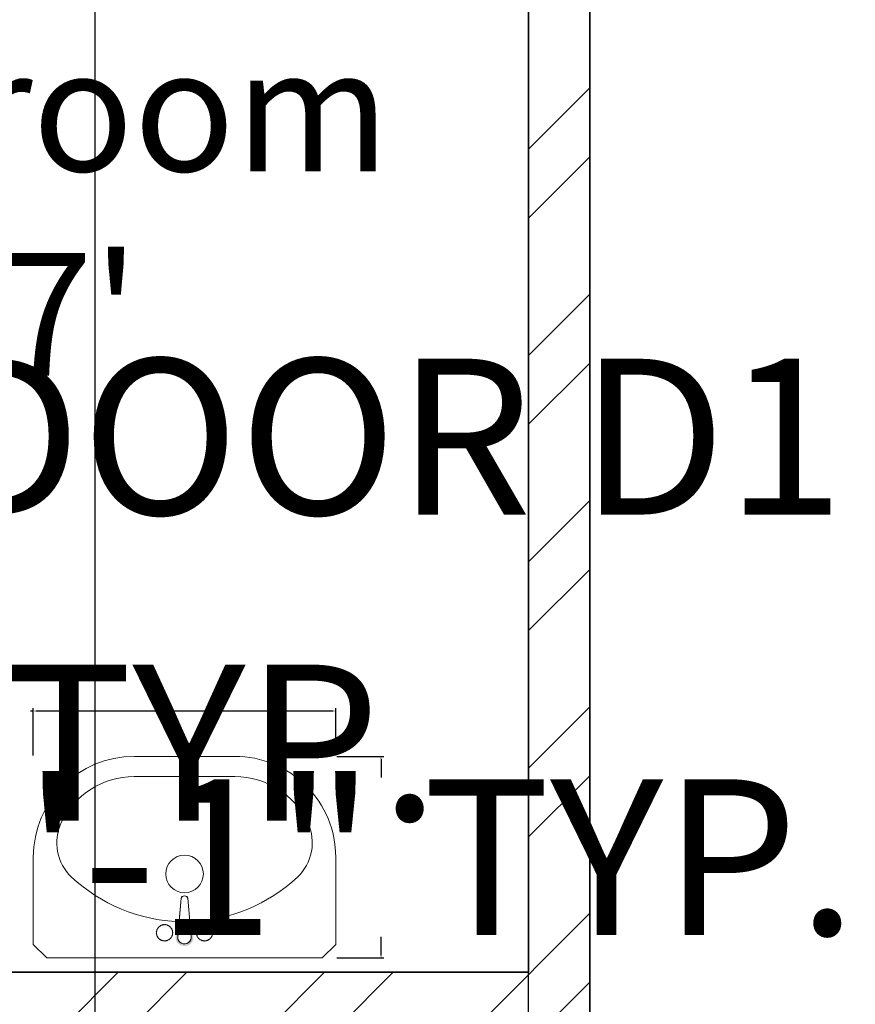
# Model space of a CAD drawing. Units: inches. Extents: x 2379 to 3013, y 1431 to 2110.
# Tile 7 of 10: x 2730 to 2785, y 1927 to 1991. Entities that reach past the tile are written whole.
import ezdxf

# ---------------------------------------------------------------- set-up
doc = ezdxf.new("R2010")
doc.units = ezdxf.units.IN
for name, color, linetype, lineweight in [('A-ANNO-DIMS', 2, 'Continuous', 18), ('A-AREA-IDEN', 7, 'Continuous', 18), ('A-FLOR-FIXT', 9, 'Continuous', 18), ('A-WALL-PATT', 8, 'Continuous', 13), ('WALL', 7, 'Continuous', 35)]:
    doc.layers.add(name, color=color, linetype=linetype, lineweight=lineweight)
doc.styles.get("Standard").update_dxf_attribs({"font": 'arial.ttf'})
doc.dimstyles.get("Standard").update_dxf_attribs({"dimtxt": 10.18, "dimasz": 0.18, "dimexe": 0.18, "dimexo": 0.0625, "dimgap": 0.09, "dimtad": 0, "dimtih": 1, "dimtoh": 1, "dimdec": 0, "dimzin": 0, "dimdsep": 46, "dimlunit": 3, "dimtxsty": 'Standard', "dimcen": 0.09, "dimadec": 0, "dimazin": 0, "dimtfac": 1, "dimtdec": 0, "dimtofl": 0, "dimtmove": 0, "dimatfit": 3, "dimfxl": 1, "dimtolj": 1, "dimtzin": 0, "dimarcsym": 0})

# ---------------------------------------------------------------- blocks, each defined once
blk = doc.blocks.new('s_46')
at = {"ltscale": 600}
h = blk.add_hatch(color=256, dxfattribs=at)
edge = h.paths.add_edge_path()
edge.add_line((13.45184378023259, 62.04360352296498), (14.15927104179718, 54.09782096462731))
edge.add_ellipse((4.212458010588306, 52.31250418393756), major_axis=(-10.10576298371302, 2.5e-15), ratio=1, start_angle=540, end_angle=550.1754626554052, ccw=False)
edge.add_arc((4.212458010588306, 52.31250418393756), 10.10576298371302, 270, 360, ccw=False)
edge.add_line((4.212458010588306, 42.20674120020703), (4.212458010588306, 41.28018079043977))
edge.add_line((4.212458010588306, 41.28018079040339), (11.85106942148559, 41.28018079040339))
edge.add_arc((4.212458010588306, 52.31250418393756), 13.41866400745597, 664.6981342835142, 766.4847699121552)
h.paths.add_polyline_path([(4.212458010588306, 41.28018079040339), (-3.426153400272596, 41.28018079040339, 0.152566653256377), (4.212458010588306, 38.8938401764608)])
h.paths.add_polyline_path([(11.85106942144921, 41.28018079040339), (4.212458010588306, 41.28018079040339), (4.212458010588306, 38.8938401764608, 0.1525666532563772)])
h.paths.add_polyline_path([(-5.734355020395014, 54.09782096461277), (-5.026927758881356, 62.04360352296498, 0.4758332592079194), (-3.426153400272596, 41.28018079040339), (4.212458010588306, 41.28018079040339), (4.212458010588306, 42.20674120020703, -0.4672400657637396)])
for p, q in [((-5.893304973142221, 52.31250418385025), (-0.714987907151226, 110.4750654234667)), ((-5.893304973142221, 52.31250418385025), (-0.714987907151226, 110.4750654234667)), ((9.139903928502463, 110.475065423554), (14.15927104174625, 54.09782096461277)), ((14.31822099431883, 52.31250418385025), (9.139903928502463, 110.475065423554)), ((14.15927104174625, 54.09782096461277), (14.31822099431883, 52.31250418385025))]:
    blk.add_line(p, q, dxfattribs=at)
blk.add_lwpolyline([(-220.7875419894117, 171.2801807903452, -0.4142135623730951), (-70.7875419894117, 321.2801807903452), (79.2124580105883, 321.2801807904325, -0.4142135623730951), (229.2124580105883, 171.2801807904325), (229.2124580105883, 41.28018079040339), (209.2124580107047, 21.2801807904325), (-200.7875419893535, 21.28018079034518), (-220.7875419894117, 41.28018079040339)], format="xyb", close=True, dxfattribs=at)
blk.add_lwpolyline([(12.26164246437838, 75.41187665969483, 0.1816379869150311), (172.1859176590806, 141.5383421540609, 0.3263505073803008), (187.6570333366981, 222.6589125997853, 0.2898144196813102), (79.21245801076293, 291.2801807904325), (-70.78754198923707, 291.2801807903452, 0.2898144196813102), (-179.2321173155214, 222.658912599698, 0.3263505073803008), (-163.7610016377293, 141.5383421540609, 0.1816379869150315), (-3.836726442852523, 75.41187665960751)], format="xyb", dxfattribs=at)
for points in [[(-16.83803374727722, 67.43055756771354), (-17.02338931558188, 67.50428807432763), (-17.22058725368697, 67.56961317334208), (-17.42189012444578, 67.6347039079701), (-17.61956049106084, 67.70773132116301), (-17.80586091603618, 67.79686645595939), (-17.97305396257434, 67.91028035557245), (-18.11578784312587, 68.05326030802098), (-18.23825336818117, 68.21955858168076), (-18.34702699835179, 68.40004368982045), (-18.44868519355077, 68.58558414605795), (-18.54980441438965, 68.76704846357461), (-18.65696112113073, 68.9353051558137), (-18.77673177386168, 69.08122273621848), (-18.91569283319404, 69.19566971814493), (-19.07841429975815, 69.27267628890695), (-19.26144033775199, 69.31891933156292), (-19.45930865121772, 69.34423740339116), (-19.66655694507062, 69.35846906132065), (-19.87772292352747, 69.37145286262967), (-20.08734429115429, 69.39302736415993), (-20.2899587523425, 69.43303112310241), (-20.48010401183274, 69.50130269664805), (-20.65391131333308, 69.60429419830325), (-20.81388605764368, 69.73491196823306), (-20.96412718523061, 69.8826759030926), (-21.10873363655992, 70.03710589953698), (-21.25180435174844, 70.18772185422131), (-21.39743827126222, 70.3240436638007), (-21.54973433539272, 70.43559122501756), (-21.71279148443137, 70.5118844343524), (-21.88955151231494, 70.54600451889564), (-22.07832762773614, 70.54527802669325), (-22.27627589285839, 70.52059283622657), (-22.4805523698451, 70.48283682571491), (-22.68831312085968, 70.44289787355228), (-22.89671420806553, 70.41166385821998), (-23.10291169380071, 70.40002265802468), (-23.30406164005399, 70.41886215136037), (-23.49802141042892, 70.4753938675276), (-23.68545357254334, 70.56212393892929), (-23.86772199510597, 70.66788214896224), (-24.04619054717477, 70.78149828102323), (-24.22222309763311, 70.89180211850908), (-24.39718351518968, 70.98762344472925), (-24.57243566872785, 71.05779204316786), (-24.74934342730558, 71.09113769704709), (-24.92903553397628, 71.08022740500746), (-25.11170022917213, 71.03257702605333), (-25.2972906283685, 70.95943963443278), (-25.48575984616764, 70.8720683044812), (-25.67706099752104, 70.7817161102721), (-25.87114719772944, 70.69963612605352), (-26.0679715613951, 70.63708142607356), (-26.26748720381875, 70.60530508466763), (-26.46941223740578, 70.61182491958607), (-26.67252476507565, 70.64921772302478), (-26.87536788737634, 70.70632503094384), (-27.07648470485583, 70.77198837930337), (-27.27441831788747, 70.8350493038015), (-27.46771182701923, 70.88434934031102), (-27.6549083327991, 70.90873002487933), (-27.83455093560042, 70.8970328932919), (-28.00620139669627, 70.84190539614065), (-28.17349611973623, 70.75121864315588), (-28.34109016874572, 70.63664965887438), (-28.51363860827405, 70.50987546765828), (-28.69579650234664, 70.38257309404435), (-28.89221891516354, 70.26641956248204), (-29.10756091127405, 70.17309189750813), (-29.3464775547036, 70.11426712348475), (-29.61160253512208, 70.0940409177856), (-29.89748404390411, 70.0861835690448), (-30.19664889771957, 70.05688401864609), (-30.50162391323829, 69.9723312081478), (-30.80493590747938, 69.79871407902101), (-31.09911169676343, 69.50222157256212), (-31.37667809793493, 69.0490426304168), (-31.63016192783834, 68.40536619405611), (-32.32050594605971, 68.4500712644367), (-32.84873653826071, 68.3918758847285), (-33.24226493795868, 68.25193804170704), (-33.52850237919483, 68.0514157223224), (-33.73486009566113, 67.8114669136994), (-33.88874932087492, 67.5532496026135), (-34.01758128887741, 67.29792177610216), (-34.14876723336056, 67.06664142102818), (-34.30371923936764, 66.87550954936887), (-34.47985279804561, 66.72039927294827), (-34.66858425136889, 66.59212672835565), (-34.86132994201034, 66.48150805244222), (-35.04950621211901, 66.37935938188457), (-35.22452940384392, 66.27649685335928), (-35.37781585985795, 66.16373660371755), (-35.50078192248475, 66.03189476963598), (-35.58785390376579, 65.87432967920904), (-35.64549799636007, 65.69456842611542), (-35.68319036299363, 65.49868029527715), (-35.7104071660433, 65.2927345718781), (-35.73662456823513, 65.08280054092756), (-35.77131873212056, 64.87494748734753), (-35.82396582007641, 64.67524469623459), (-35.90404199482873, 64.48976145259803), (-36.01774371694773, 64.3227640100813), (-36.15814863995183, 64.17130649695173), (-36.31505471485434, 64.0306400101108), (-36.47825989319244, 63.89601564637269), (-36.63756212632871, 63.76268450255157), (-36.78275936545106, 63.62589767554891), (-36.90364956192207, 63.48090626226621), (-36.99003066710429, 63.32296135951764), (-37.03518227743916, 63.14869254492805), (-37.04631056915969, 62.96024331927765), (-37.03410336375237, 62.7611356638954), (-37.00924848217983, 62.55489156045951), (-36.98243374592858, 62.34503299021162), (-36.96434697631048, 62.13508193491725), (-36.96567599463743, 61.92856037581805), (-36.99710862222128, 61.72899029450491), (-37.06570762058254, 61.53896291530691), (-37.16403551277472, 61.35734643402975), (-37.28102976223454, 61.18207828939194), (-37.40562783187488, 61.0110959201993), (-37.52676718513249, 60.84233676508302), (-37.63338528544409, 60.67373826284892), (-37.7144195958972, 60.50323785204091), (-37.75880757992855, 60.32877297155209), (-37.75920177751686, 60.14875038337777), (-37.72311503690435, 59.96345414296957), (-37.66177528270055, 59.77363762940512), (-37.58641044021351, 59.58005422132555), (-37.5082484340528, 59.38345729780849), (-37.43851718935184, 59.18460023758234), (-37.38844463089481, 58.98423641963745), (-37.36925868364051, 58.78311922278953), (-37.38844463089481, 58.58200202594161), (-37.43851718935184, 58.38163820799673), (-37.5082484340528, 58.18278114777058), (-37.58641044021351, 57.98618422425352), (-37.66177528287517, 57.79260081626126), (-37.72311503690435, 57.6027843026095), (-37.75920177751686, 57.4174880622013), (-37.75880757992855, 57.23746547402697), (-37.7144195958972, 57.06300059353816), (-37.63338528544409, 56.89250018273014), (-37.52676718530711, 56.72390168049606), (-37.40562783187488, 56.55514252537978), (-37.28102976223454, 56.38416015618713), (-37.16403551277472, 56.20889201154932), (-37.06570762058254, 56.02727553035947), (-36.99710862222128, 55.83724815107416), (-36.96567599463743, 55.63767806976102), (-36.96434697631048, 55.43115651066182), (-36.98243374592858, 55.22120545536745), (-37.00924848217983, 55.01134688520687), (-37.03410336375237, 54.80510278168367), (-37.04631056933431, 54.60599512638873), (-37.03518227743916, 54.41754590065102), (-36.99003066710429, 54.24327708606142), (-36.90364956192207, 54.08533218331285), (-36.78275936545106, 53.94034077003016), (-36.63756212632871, 53.80355394302751), (-36.47825989319244, 53.67022279920639), (-36.31505471502896, 53.53559843546827), (-36.15814863995183, 53.39493194862734), (-36.01774371712236, 53.24347443549777), (-35.90404199482873, 53.07647699298104), (-35.82396582007641, 52.89099374934449), (-35.77131873212056, 52.69129095823155), (-35.73662456823513, 52.48343790465151), (-35.71040716621792, 52.27350387370098), (-35.68319036299363, 52.06755815021461), (-35.64549799653469, 51.87167001946363), (-35.58785390376579, 51.69190876637003), (-35.50078192248475, 51.53434367594309), (-35.3778353385278, 51.40284301002975), (-35.22468523163116, 51.29247093791491), (-35.05003213009331, 51.19609060572111), (-34.86257656256203, 51.10656515930895), (-34.67101905716118, 51.01675774488831), (-34.48406014236389, 50.91953150840708), (-34.31040034646867, 50.80774959607516), (-34.15874019777402, 50.67427515375311), (-34.03505195630714, 50.51453334218241), (-33.93439480883535, 50.3341973797942), (-33.84909967368003, 50.14150249981321), (-33.77149746881332, 49.94468393520219), (-33.69391911290586, 49.75197691909852), (-33.60869552427903, 49.57161668455228), (-33.50815762107959, 49.41183846470085), (-33.38463632145431, 49.28087749250699), (-33.23284944484476, 49.18408373402781), (-33.05706241185544, 49.11526608630083), (-32.86392754490953, 49.06534817945794), (-32.66009716555709, 49.02525364354369), (-32.45222359569743, 48.98590610860265), (-32.24695915722987, 48.93822920459206), (-32.05095617187908, 48.87314656155649), (-31.870866961719, 48.78158180962782), (-31.71133844077122, 48.65761859554914), (-31.5689958925941, 48.50798063381808), (-31.43845919286832, 48.34255165536887), (-31.31434821744915, 48.17121539139771), (-31.19128284219187, 48.00385557310073), (-31.06388294277713, 47.85035593167413), (-30.92676839523483, 47.72060019822674), (-30.77455907507101, 47.62447210386745), (-30.60346923320321, 47.56846716045401), (-30.41609062027419, 47.54552800310193), (-30.21660936163971, 47.54520904741366), (-30.00921158283018, 47.55706470907898), (-29.79808340937598, 47.570649403875), (-29.58741096680751, 47.57551754757878), (-29.38138038065517, 47.56122355579281), (-29.18417777627474, 47.51732184420689), (-28.99883273948217, 47.43692629240103), (-28.8237486963626, 47.32738863455597), (-28.65617253311211, 47.19962006882997), (-28.49335113610141, 47.06453179311938), (-28.33253139152657, 46.9330350055825), (-28.1709601857583, 46.81604090429027), (-28.00588440499268, 46.72446068713907), (-27.83455093577504, 46.66920555219985), (-27.6549083327991, 46.65750842061243), (-27.46771182701923, 46.68188910518074), (-27.27441831788747, 46.73118914177758), (-27.07648470485583, 46.7942500662757), (-26.87536788755096, 46.85991341454792), (-26.67252476525027, 46.91702072246698), (-26.4694122375804, 46.95441352590569), (-26.26748720399337, 46.96093336082412), (-26.06797156156972, 46.9291570194182), (-25.87114719772944, 46.86660231943824), (-25.67706099769566, 46.78452233530697), (-25.48575984616764, 46.69417014101054), (-25.2972906283685, 46.60679881105898), (-25.11170022934675, 46.53366141943843), (-24.92903553397628, 46.4860110404843), (-24.74934342730558, 46.47510074844467), (-24.57243566890247, 46.50844640232389), (-24.39718351536431, 46.57861500076251), (-24.22222309780773, 46.67443632698268), (-24.0461905473494, 46.78474016446853), (-23.86772199528059, 46.89835629652953), (-23.68545357254334, 47.00411450656247), (-23.49802141060354, 47.09084457796416), (-23.30406164022861, 47.14737629413138), (-23.10291169380071, 47.16621578746708), (-22.89671420806553, 47.15457458727178), (-22.68831312085968, 47.12334057193948), (-22.4805523698451, 47.08340161977685), (-22.27627589285839, 47.04564560926519), (-22.07832762791077, 47.02096041871118), (-21.88955151248956, 47.02023392650881), (-21.71279148443137, 47.05435401113937), (-21.54973433539272, 47.1306472204742), (-21.39743827126222, 47.24219478160375), (-21.25180435174844, 47.37851659118314), (-21.10873363655992, 47.52913254586746), (-20.96412718540523, 47.68356254231185), (-20.81388605764368, 47.83132647717138), (-20.65391131333308, 47.9619442471012), (-20.48010401200736, 48.0649357488437), (-20.28995875251712, 48.13320732230204), (-20.08734429115429, 48.17321108133183), (-19.87772292352747, 48.1947855828621), (-19.66655694507062, 48.2077693840838), (-19.45930865139235, 48.2220010421006), (-19.26144033775199, 48.24731911384152), (-19.07841429993277, 48.29356215667212), (-18.91569283319404, 48.37056872743414), (-18.77673177403631, 48.48501570936059), (-18.65696112113073, 48.63093328976538), (-18.54980441456428, 48.79918998200446), (-18.44868519372539, 48.98065429960843), (-18.34702699835179, 49.16619475575862), (-18.2382533683558, 49.34667986398562), (-18.11578784312587, 49.5129781376454), (-17.97305396274896, 49.6559580900066), (-17.8058609162108, 49.76937198961969), (-17.61956049106084, 49.85850712450337), (-17.4218901246204, 49.93153453769628), (-17.22058725368697, 49.996625272237), (-17.02338931558188, 50.06195037133875), (-16.83803374727722, 50.13568087795284), (-16.67225798609434, 50.22598783511785), (-16.53379946883069, 50.34104228604701), (-16.42766593385022, 50.48645191569812), (-16.34794632298872, 50.65757097714231), (-16.28599987912457, 50.84719036528259), (-16.23318584513618, 51.04810097528389), (-16.18086346407654, 51.25309370196191), (-16.12039197882404, 51.45495944039431), (-16.04313063243171, 51.64648908557137), (-15.94043866742868, 51.82047353248345), (-15.8067031877581, 51.97190354572376), (-15.64842273970134, 52.10456936812261), (-15.47512373042991, 52.22446111202589), (-15.29633256676607, 52.33756888969219), (-15.12157565605594, 52.44988281364204), (-14.96037940529641, 52.567392996134), (-14.82227022130973, 52.69608954960131), (-14.71677451161667, 52.84196258638985), (-14.6501372611965, 53.00919824198354), (-14.61547776852967, 53.19476674450561), (-14.60263391025364, 53.3938343450427), (-14.60144356318051, 53.60156729485606), (-14.60174460412236, 53.81313184503233), (-14.59337490954203, 54.02369424700736), (-14.566172356077, 54.22842075169319), (-14.50997482053935, 54.42247761052567), (-14.41809999983525, 54.6024088327249), (-14.29778487142175, 54.77026946117985), (-14.1597462335485, 54.92949229647638), (-14.01470088359201, 55.08351013963693), (-13.87336561962729, 55.23575579150929), (-13.7464572393801, 55.38966205302859), (-13.64469254092546, 55.54866172495531), (-13.5787883218145, 55.71618760822457), (-13.55583441938506, 55.89474125843844), (-13.56841282837558, 56.08309925056528), (-13.60547858278733, 56.27910691397847), (-13.65598671662155, 56.48060957840062), (-13.70889226370491, 56.68545257346704), (-13.7531502583879, 56.89148122872575), (-13.7777157346718, 57.09654087381204), (-13.77154372638324, 57.29847683827393), (-13.72730239736847, 57.49560352915432), (-13.65251243085367, 57.68811166286468), (-13.55840763938613, 57.8766610333987), (-13.45622183586238, 58.06191143448813), (-13.35718883317895, 58.24452266012667), (-13.27254244388314, 58.42515450413339), (-13.2135164810461, 58.60446676041465), (-13.19134475721512, 58.78311922278953), (-13.2135164810461, 58.96177168516442), (-13.27254244388314, 59.14108394144569), (-13.35718883317895, 59.3217157854524), (-13.45622183586238, 59.50432701109093), (-13.55840763938613, 59.68957741218037), (-13.65251243085367, 59.87812678271438), (-13.72730239736847, 60.07063491642475), (-13.77154372638324, 60.26776160730515), (-13.7777157346718, 60.46969757176703), (-13.7531502583879, 60.67475721685332), (-13.70889226370491, 60.88078587211203), (-13.65598671662155, 61.08562886717845), (-13.60547858278733, 61.2871315316006), (-13.56841282837558, 61.48313919501379), (-13.55583441938506, 61.67149718714063), (-13.5787883218145, 61.8500508373545), (-13.64469254092546, 62.01757672062377), (-13.7464572393801, 62.17657639255048), (-13.87336561962729, 62.33048265406978), (-14.01470088359201, 62.48272830594214), (-14.15974623337388, 62.63674614910269), (-14.29778487142175, 62.79596898448653), (-14.41809999983525, 62.96382961285416), (-14.50997482053935, 63.14376083514071), (-14.566172356077, 63.33781769388588), (-14.59337490936741, 63.5425441985717), (-14.60174460412236, 63.75310660054674), (-14.60144356318051, 63.96467115081032), (-14.60263391025364, 64.17240410053635), (-14.61547776835505, 64.37147170116077), (-14.65013726102188, 64.55704020359553), (-14.71677451144205, 64.7242758591892), (-14.82227022130973, 64.87014889597776), (-14.96037940529641, 64.99884544944507), (-15.12157565605594, 65.11635563193704), (-15.29633256676607, 65.22866955588688), (-15.47512373042991, 65.3417773336405), (-15.64842273970134, 65.46166907745646), (-15.8067031877581, 65.59433489985531), (-15.94043866742868, 65.74576491309563), (-16.04313063225709, 65.9197493600077), (-16.12039197882404, 66.11127900527208), (-16.18086346407654, 66.31314474370447), (-16.23318584513618, 66.5181374703825), (-16.28599987912457, 66.71904808029649), (-16.34794632298872, 66.90866746843676), (-16.42766593385022, 67.07978652988095), (-16.53379946883069, 67.22519615953206), (-16.67225798609434, 67.34025061046123)], [(22.08090273779817, 61.08562886709115), (22.03039460413856, 61.2871315315133), (21.99332884972682, 61.48313919501379), (21.9807504407363, 61.67149718705331), (22.00370434316574, 61.85005083726719), (22.06960856210208, 62.01757672053645), (22.17137326073134, 62.17657639246318), (22.29828164080391, 62.33048265398247), (22.43961690476863, 62.48272830585483), (22.58466225472512, 62.63674614901538), (22.72270089277299, 62.79596898439923), (22.84301602118649, 62.96382961276686), (22.93489084189059, 63.1437608350534), (22.99108837742824, 63.33781769379857), (23.01829093071865, 63.5425441985717), (23.0266606254736, 63.75310660045943), (23.02635958453175, 63.96467115072301), (23.02754993160488, 64.17240410053635), (23.04039378970629, 64.37147170107346), (23.07505328237312, 64.55704020350822), (23.14169053279329, 64.72427585910191), (23.24718624266097, 64.87014889589045), (23.38529542664764, 64.99884544935776), (23.54649167740717, 65.11635563193704), (23.7212485881173, 65.22866955579956), (23.90003975178115, 65.34177733355318), (24.07333876105258, 65.46166907736915), (24.23161920910934, 65.594334899768), (24.36535468877992, 65.74576491300832), (24.46804665360833, 65.9197493600077), (24.54530800017528, 66.11127900518477), (24.60577948542777, 66.31314474361714), (24.65810186648742, 66.51813747029519), (24.71091590047581, 66.71904808020918), (24.77286234433996, 66.90866746834945), (24.85258195520146, 67.07978652979364), (24.95871549018193, 67.22519615953206), (25.09717400744558, 67.34025061046123), (25.26294976862846, 67.43055756771354), (25.44830533693312, 67.50428807432763), (25.64550327503821, 67.56961317334208), (25.84680614579702, 67.6347039079701), (26.04447651241208, 67.70773132116301), (26.23077693756204, 67.79686645595939), (26.3979699841002, 67.91028035557245), (26.54070386447711, 68.05326030802098), (26.66316938970704, 68.21955858168076), (26.77194301970303, 68.40004368982045), (26.87360121507663, 68.58558414605795), (26.97472043591552, 68.76704846357461), (27.08187714248197, 68.9353051558137), (27.20164779538754, 69.08122273621848), (27.34060885454528, 69.19566971814493), (27.50333032128401, 69.27267628890695), (27.68635635910323, 69.31891933165025), (27.88422467274358, 69.34423740347847), (28.09147296642186, 69.35846906140794), (28.30263894487871, 69.37145286262967), (28.51226031250553, 69.39302736424725), (28.71487477386836, 69.43303112318972), (28.90502003318398, 69.50130269673537), (29.07882733468432, 69.60429419839056), (29.23880207899492, 69.73491196832038), (29.38904320658185, 69.88267590317992), (29.53364965791116, 70.0371058996243), (29.67672037309967, 70.18772185430862), (29.82235429261346, 70.324043663888), (29.97465035674395, 70.43559122501756), (30.1377075057826, 70.51188443443971), (30.31446753366618, 70.54600451898295), (30.50324364908738, 70.54527802678058), (30.70119191420963, 70.52059283622657), (30.90546839119634, 70.48283682571491), (31.11322914221091, 70.4428978736396), (31.32163022941677, 70.41166385830729), (31.52782771515195, 70.400022658112), (31.72897766157985, 70.41886215144768), (31.92293743178016, 70.4753938675276), (32.11036959389458, 70.56212393892929), (32.29263801663183, 70.66788214896224), (32.47110656870063, 70.78149828102323), (32.64713911898434, 70.89180211850908), (32.82209953654092, 70.98762344481656), (32.99735169025371, 71.05779204316786), (33.17425944865681, 71.09113769704709), (33.35395155532751, 71.08022740500746), (33.53661625069799, 71.03257702605333), (33.72220664971974, 70.9594396345201), (33.91067586751888, 70.8720683044812), (34.1019770190469, 70.7817161102721), (34.29606321908068, 70.69963612605352), (34.49288758292096, 70.63708142616088), (34.69240322534461, 70.60530508466763), (34.89432825893164, 70.61182491958607), (35.09744078660151, 70.64921772302478), (35.3002839089022, 70.70632503103116), (35.50140072620707, 70.77198837930337), (35.6993343392387, 70.8350493038015), (35.89262784837047, 70.88434934039833), (36.07982435415034, 70.90873002487933), (36.25946695695166, 70.8970328932919), (36.43111741804751, 70.84190539614065), (36.59841214108747, 70.75121864315588), (36.76600619009696, 70.63664965887438), (36.93855462962529, 70.50987546765828), (37.12071252369788, 70.38257309404435), (37.3171349366894, 70.26641956248204), (37.53247693262529, 70.17309189750813), (37.77139357605483, 70.11426712348475), (38.03651855647331, 70.0940409177856), (38.32240006525535, 70.0861835690448), (38.62156491907081, 70.05688401864609), (38.92653993476415, 69.9723312081478), (39.22985192883061, 69.79871407893368), (39.52402771811467, 69.50222157256212), (39.80159411928616, 69.0490426304168), (40.05507794918957, 68.4053661939688), (40.74542196741094, 68.4500712644367), (41.27365255961194, 68.3918758846412), (41.66718095948453, 68.25193804161972), (41.95341840054607, 68.0514157223224), (42.15977611701236, 67.8114669136121), (42.31366534240078, 67.5532496025262), (42.44249731022864, 67.29792177601485), (42.57368325471179, 67.06664142094087), (42.72863526071887, 66.87550954936887), (42.90476881939684, 66.72039927286096), (43.09350027272012, 66.59212672826834), (43.28624596336157, 66.48150805235491), (43.47442223347025, 66.37935938179726), (43.64944542536977, 66.27649685335928), (43.80273188138381, 66.16373660371755), (43.92569794383598, 66.03189476963598), (44.01276992511703, 65.87432967912173), (44.0704140177113, 65.69456842602813), (44.10810638434486, 65.49868029527715), (44.13532318739453, 65.2927345718781), (44.16154058958636, 65.08280054084025), (44.19623475347179, 64.87494748726021), (44.24888184142765, 64.67524469614727), (44.32895801617997, 64.48976145251072), (44.44265973829897, 64.32276400999397), (44.58306466130307, 64.17130649695173), (44.73997073620558, 64.03064001002348), (44.90317591454368, 63.89601564628538), (45.06247814767994, 63.76268450246425), (45.20767538680229, 63.6258976754616), (45.3285655832733, 63.4809062621789), (45.41494668845553, 63.32296135943034), (45.46009829879039, 63.14869254484074), (45.47122659051092, 62.96024331919034), (45.45901938492898, 62.76113566380809), (45.43416450353106, 62.5548915603722), (45.40734976727981, 62.34503299021162), (45.38926299766171, 62.13508193482994), (45.39059201598866, 61.92856037573074), (45.42202464357251, 61.7289902944176), (45.49062364193377, 61.53896291521959), (45.58895153412595, 61.35734643394243), (45.70594578341115, 61.18207828939194), (45.83054385322611, 61.01109592011198), (45.95168320648371, 60.84233676508302), (46.05830130679533, 60.67373826276162), (46.13933561724843, 60.50323785204091), (46.18372360127978, 60.32877297146479), (46.1841177988681, 60.14875038329046), (46.14803105825558, 59.96345414296957), (46.08669130405178, 59.77363762931782), (46.01132646156474, 59.58005422123824), (45.93316445540404, 59.38345729772118), (45.86343321070308, 59.18460023749503), (45.81336065224604, 58.98423641955014), (45.79417470499175, 58.78311922270222), (45.81336065224604, 58.58200202585431), (45.86343321070308, 58.38163820790942), (45.93316445540404, 58.18278114777058), (46.01132646156474, 57.98618422416621), (46.08669130405178, 57.79260081617394), (46.14803105808095, 57.6027843025222), (46.1841177988681, 57.4174880622013), (46.18372360127978, 57.23746547393966), (46.13933561724843, 57.06300059345085), (46.05830130679533, 56.89250018273014), (45.95168320648371, 56.72390168040874), (45.83054385322611, 56.55514252529247), (45.70594578341115, 56.38416015609982), (45.58895153412595, 56.20889201154932), (45.49062364193377, 56.02727553027216), (45.42202464339789, 55.83724815107416), (45.39059201598866, 55.63767806976102), (45.38926299766171, 55.43115651066182), (45.40734976727981, 55.22120545528014), (45.43416450335644, 55.01134688511957), (45.45901938492898, 54.80510278159636), (45.47122659051092, 54.60599512630142), (45.46009829879039, 54.41754590056371), (45.41494668845553, 54.24327708597411), (45.32856558309868, 54.08533218322554), (45.20767538662767, 53.94034076994285), (45.06247814750532, 53.8035539429402), (44.90317591454368, 53.67022279920639), (44.73997073620558, 53.53559843538096), (44.58306466130307, 53.39493194854004), (44.44265973829897, 53.24347443541046), (44.32895801617997, 53.07647699298104), (44.24888184125302, 52.89099374934449), (44.19623475329717, 52.69129095823155), (44.16154058958636, 52.48343790465151), (44.13532318739453, 52.27350387361366), (44.10810638434486, 52.06755815021461), (44.0704140177113, 51.87167001946363), (44.01276992511703, 51.69190876628272), (43.92569794366136, 51.53434367585578), (43.80275135970442, 51.40284301002975), (43.64960125280776, 51.29247093791491), (43.47494815144455, 51.1960906056338), (43.28749258373863, 51.10656515922165), (43.09593507851241, 51.01675774480099), (42.90897616371512, 50.91953150840708), (42.73531636764528, 50.80774959598784), (42.58365621895063, 50.67427515375311), (42.45996797765838, 50.51453334218241), (42.35931083018658, 50.3341973797942), (42.27401569485664, 50.14150249981321), (42.19641349016455, 49.94468393520219), (42.1188351342571, 49.75197691909852), (42.03361154545564, 49.57161668455228), (41.9330736422562, 49.41183846461354), (41.80955234280554, 49.28087749250699), (41.65776546602137, 49.1840837339405), (41.48197843320668, 49.11526608630083), (41.28884356608614, 49.06534817945794), (41.0850131867337, 49.02525364354369), (40.87713961687405, 48.98590610851534), (40.67187517840648, 48.93822920459206), (40.47587219323031, 48.87314656155649), (40.29578298289561, 48.78158180962782), (40.13625446194782, 48.65761859554914), (39.99391191377072, 48.50798063373076), (39.86337521404493, 48.34255165528157), (39.73926423862577, 48.17121539139771), (39.61619886336848, 48.00385557310073), (39.48879896395374, 47.85035593167413), (39.35168441641144, 47.72060019813944), (39.19947509624762, 47.62447210378013), (39.02838525455445, 47.56846716045401), (38.8410066414508, 47.54552800310193), (38.64152538281633, 47.54520904732635), (38.43412760400679, 47.55706470907898), (38.22299943072721, 47.570649403875), (38.01232698798413, 47.57551754757878), (37.80629640183179, 47.56122355579281), (37.60909379745135, 47.51732184420689), (37.42374876065878, 47.43692629240103), (37.24866471753922, 47.32738863455597), (37.08108855428873, 47.19962006882997), (36.91826715727803, 47.06453179311938), (36.75744741270319, 46.9330350056698), (36.59587620693492, 46.81604090429027), (36.4308004261693, 46.72446068713907), (36.25946695695166, 46.66920555228716), (36.07982435397571, 46.65750842061243), (35.89262784837047, 46.68188910518074), (35.6993343392387, 46.73118914177758), (35.50140072620707, 46.7942500662757), (35.30028390872758, 46.85991341454792), (35.09744078642689, 46.91702072246698), (34.89432825875701, 46.954413525993), (34.69240322516998, 46.96093336082412), (34.49288758274633, 46.9291570194182), (34.29606321908068, 46.86660231943824), (34.10197701887228, 46.78452233530697), (33.91067586734425, 46.69417014109785), (33.72220664971974, 46.60679881105898), (33.53661625052337, 46.53366141943843), (33.35395155515289, 46.4860110404843), (33.17425944865681, 46.47510074844467), (32.99735169007909, 46.5084464024112), (32.82209953654092, 46.57861500076251), (32.64713911898434, 46.67443632707), (32.47110656852601, 46.78474016446853), (32.2926380164572, 46.89835629661684), (32.11036959389458, 47.00411450664979), (31.92293743178016, 47.09084457805147), (31.72897766140522, 47.14737629413138), (31.52782771497732, 47.16621578746708), (31.32163022941677, 47.15457458727178), (31.11322914203629, 47.12334057193948), (30.90546839102171, 47.08340161986416), (30.70119191420963, 47.0456456093525), (30.50324364908738, 47.02096041879849), (30.31446753366618, 47.02023392659611), (30.1377075057826, 47.05435401113937), (29.97465035674395, 47.13064722056151), (29.82235429261346, 47.24219478169106), (29.67672037309967, 47.37851659127045), (29.53364965791116, 47.52913254595478), (29.38904320658185, 47.68356254239916), (29.2388020788203, 47.8313264772587), (29.0788273345097, 47.96194424718851), (28.90502003318398, 48.06493574893102), (28.71487477369374, 48.13320732238935), (28.51226031250553, 48.17321108133183), (28.30263894487871, 48.19478558294941), (28.09147296642186, 48.20776938417111), (27.88422467256896, 48.22200104218791), (27.68635635892861, 48.24731911392882), (27.50333032110939, 48.29356215667212), (27.34060885454528, 48.37056872743414), (27.20164779521292, 48.48501570936059), (27.08187714248197, 48.63093328976538), (26.97472043574089, 48.79918998200446), (26.87360121490201, 48.98065429960843), (26.77194301952841, 49.16619475575862), (26.66316938953241, 49.34667986398562), (26.54070386447711, 49.51297813755809), (26.39796998392558, 49.6559580900066), (26.23077693738742, 49.76937198961969), (26.04447651223745, 49.85850712450337), (25.84680614579702, 49.93153453769628), (25.64550327486359, 49.996625272237), (25.44830533675849, 50.06195037133875), (25.26294976862846, 50.13568087795284), (25.09717400727095, 50.22598783520516), (24.95871549018193, 50.34104228604701), (24.85258195520146, 50.48645191561082), (24.77286234416534, 50.657570977055), (24.71091590030119, 50.84719036519527), (24.65810186648742, 51.04810097519657), (24.60577948542777, 51.2530937018746), (24.54530800017528, 51.45495944030699), (24.46804665360833, 51.64648908548406), (24.36535468877992, 51.82047353239614), (24.23161920910934, 51.97190354572376), (24.07333876105258, 52.1045693680353), (23.90003975160653, 52.22446111193858), (23.7212485881173, 52.33756888960488), (23.54649167740717, 52.44988281355472), (23.38529542647302, 52.56739299604669), (23.24718624266097, 52.696089549514), (23.14169053279329, 52.84196258630254), (23.07505328237312, 53.00919824189623), (23.04039378970629, 53.1947667444183), (23.02754993160488, 53.39383434495539), (23.02635958453175, 53.60156729476876), (23.02666062529898, 53.81313184503233), (23.01829093071865, 54.02369424692006), (22.99108837725362, 54.22842075169319), (22.93489084171597, 54.42247761043836), (22.84301602101186, 54.6024088327249), (22.72270089277299, 54.77026946109254), (22.58466225472512, 54.92949229638907), (22.43961690476863, 55.08351013963693), (22.29828164080391, 55.23575579150929), (22.17137326073134, 55.38966205294127), (22.06960856210208, 55.548661724868), (22.00370434316574, 55.71618760813726), (21.9807504407363, 55.89474125843844), (21.99332884972682, 56.08309925047797), (22.03039460413856, 56.27910691389115), (22.08090273779817, 56.48060957840062), (22.13380828505615, 56.68545257346704), (22.17806627973914, 56.89148122872575), (22.20263175602304, 57.09654087381204), (22.19645974773448, 57.29847683827393), (22.15221841871971, 57.49560352915432), (22.07742845220491, 57.68811166286468), (21.98332366073737, 57.87666103331139), (21.88113785721362, 58.06191143448813), (21.78210485453019, 58.24452266012667), (21.69745846523438, 58.42515450413339), (21.63843250239734, 58.60446676032734), (21.61626077856636, 58.78311922270222), (21.63843250239734, 58.96177168507711), (21.69745846523438, 59.14108394135837), (21.78210485453019, 59.32171578536508), (21.88113785721362, 59.50432701100362), (21.98332366073737, 59.68957741209306), (22.07742845220491, 59.87812678262708), (22.15221841871971, 60.07063491633743), (22.19645974773448, 60.26776160721784), (22.20263175602304, 60.46969757167971), (22.17806627973914, 60.67475721676601), (22.13380828505615, 60.88078587202471)]]:
    blk.add_lwpolyline(points, close=True, dxfattribs=at)
blk.add_circle((4.212458010588306, 146.2801807904034), 28, dxfattribs=at)
for centre, radius, start, end in [((4.212458010588306, 108.2109541267855), 5.422722861947412, 24.67830004152974, 155.3216999584702), ((4.212458010588306, 52.31250418393756), 10.10576298371233, 169.8245373479931, 0)]:
    blk.add_arc(centre, radius, start, end, dxfattribs=at)
for centre, major_axis, ratio, start_param, end_param in [((4.212458010762929, 110.475065423554), (-4.927445917859709, 1.2e-15), 0.6410240960233505, 3.141592653589793, 6.283185307179586), ((4.212458010588306, 52.31250418393756), (-10.10576298371302, 2.5e-15), 1, 6.105589980929039, 9.602373287019926)]:
    blk.add_ellipse(centre, major_axis=major_axis, ratio=ratio, start_param=start_param, end_param=end_param, dxfattribs=at)
blk = doc.blocks.new('*D26')
at = {"layer": 'A-ANNO-DIMS', "color": 0, "lineweight": -2, "transparency": 16777216}
for p, q in [((2688.622898699378, 1958.67097978589), (2688.622898699378, 1963.759108581785)), ((2688.802898699378, 1963.579108581785), (2721.580424005343, 1963.579108581785)), ((2721.760424005343, 1958.67097978589), (2721.760424005343, 1963.759108581785)), ((2721.760424005343, 1963.579108581785), (2721.940424005343, 1963.579108581785))]:
    blk.add_line(p, q, dxfattribs=at)
at = {"layer": 'A-ANNO-DIMS', "color": 0, "transparency": 16777216}
for points in [[(2688.802898699378, 1963.609108581785), (2688.802898699378, 1963.549108581785), (2688.622898699378, 1963.579108581785)], [(2721.580424005343, 1963.609108581785), (2721.580424005343, 1963.549108581785), (2721.760424005343, 1963.579108581785)]]:
    blk.add_solid(points, dxfattribs=at)
at = {"layer": 'Defpoints', "color": 0, "transparency": 16777216}
for p in [(2721.760424005343, 1963.579108581785), (2688.622898699378, 1958.60847978589), (2721.760424005343, 1958.60847978589)]:
    blk.add_point(p, dxfattribs=at)
at = {"layer": 'A-ANNO-DIMS', "color": 0, "transparency": 16777216, "insert": (2787.176174346408, 1963.579108581785), "char_height": 10.18, "attachment_point": 5}
blk.add_mtext('\\A1;DOOR D1 2\'-9" TYP.', dxfattribs=at)
blk = doc.blocks.new('*D27')
at = {"layer": 'A-ANNO-DIMS', "color": 0, "lineweight": -2, "transparency": 16777216}
for p, q in [((2721.822924005344, 1958.608479785891), (2726.91105280124, 1958.608479785891)), ((2726.73105280124, 1958.428479785891), (2726.73105280124, 1948.896112800894)), ((2726.73105280124, 1928.788479785884), (2726.73105280124, 1938.320846770881)), ((2721.822924005344, 1928.608479785884), (2726.91105280124, 1928.608479785884))]:
    blk.add_line(p, q, dxfattribs=at)
at = {"layer": 'A-ANNO-DIMS', "color": 0, "transparency": 16777216}
for points in [[(2726.701052801239, 1958.428479785891), (2726.76105280124, 1958.428479785891), (2726.73105280124, 1958.608479785891)], [(2726.701052801239, 1928.788479785884), (2726.76105280124, 1928.788479785884), (2726.73105280124, 1928.608479785884)]]:
    blk.add_solid(points, dxfattribs=at)
at = {"layer": 'Defpoints', "color": 0, "transparency": 16777216}
for p in [(2721.760424005344, 1958.608479785891), (2721.760424005344, 1928.608479785884), (2726.73105280124, 1928.608479785884)]:
    blk.add_point(p, dxfattribs=at)
at = {"layer": 'A-ANNO-DIMS', "color": 0, "transparency": 16777216, "insert": (2726.73105280124, 1943.608479785886), "char_height": 10.18, "attachment_point": 5}
blk.add_mtext('\\A1;2\'-6" TYP.', dxfattribs=at)
blk = doc.blocks.new('*D42')
at = {"layer": 'A-ANNO-DIMS', "color": 0, "lineweight": -2, "transparency": 16777216}
for p, q in [((2731.292496124008, 1945.667853308336), (2731.112496124008, 1945.667853308336)), ((2731.292496124008, 1942.76850560317), (2731.292496124008, 1945.847853308336)), ((2750.858147491776, 1945.667853308336), (2731.472496124008, 1945.667853308336)), ((2751.038147491776, 1942.76850560317), (2751.038147491776, 1945.847853308336))]:
    blk.add_line(p, q, dxfattribs=at)
at = {"layer": 'A-ANNO-DIMS', "color": 0, "transparency": 16777216}
for points in [[(2731.472496124008, 1945.697853308336), (2731.472496124008, 1945.637853308335), (2731.292496124008, 1945.667853308336)], [(2750.858147491776, 1945.697853308336), (2750.858147491776, 1945.637853308335), (2751.038147491776, 1945.667853308336)]]:
    blk.add_solid(points, dxfattribs=at)
at = {"layer": 'Defpoints', "color": 0, "transparency": 16777216}
for p in [(2731.292496124008, 1945.667853308336), (2731.292496124008, 1942.70600560317), (2751.038147491776, 1942.70600560317)]:
    blk.add_point(p, dxfattribs=at)
at = {"layer": 'A-ANNO-DIMS', "color": 0, "transparency": 16777216, "insert": (2665.046929957569, 1945.667853308336), "char_height": 10.18, "attachment_point": 5}
blk.add_mtext('\\A1;BASIN 1\'-7 1/2" TYP.', dxfattribs=at)
blk = doc.blocks.new('*D43')
at = {"layer": 'A-ANNO-DIMS', "color": 0, "lineweight": -2, "transparency": 16777216}
for p, q in [((2751.100647491777, 1942.706005603171), (2754.179995196943, 1942.706005603171)), ((2753.999995196943, 1942.526005603171), (2753.999995196943, 1941.328426043108)), ((2753.999995196943, 1929.722238024655), (2753.999995196943, 1930.919817584718)), ((2751.100647491777, 1929.542238024655), (2754.179995196943, 1929.542238024655))]:
    blk.add_line(p, q, dxfattribs=at)
at = {"layer": 'A-ANNO-DIMS', "color": 0, "transparency": 16777216}
for points in [[(2753.969995196943, 1942.526005603171), (2754.029995196944, 1942.526005603171), (2753.999995196943, 1942.706005603171)], [(2753.969995196943, 1929.722238024655), (2754.029995196944, 1929.722238024655), (2753.999995196943, 1929.542238024655)]]:
    blk.add_solid(points, dxfattribs=at)
at = {"layer": 'Defpoints', "color": 0, "transparency": 16777216}
for p in [(2751.038147491777, 1942.706005603171), (2753.999995196943, 1942.706005603171), (2751.038147491777, 1929.542238024655)]:
    blk.add_point(p, dxfattribs=at)
at = {"layer": 'A-ANNO-DIMS', "color": 0, "transparency": 16777216, "insert": (2753.999995196943, 1936.124121813912), "char_height": 10.18, "attachment_point": 5}
blk.add_mtext('\\A1;1\'-1" TYP.', dxfattribs=at)
blk = doc.blocks.new('*D46')
at = {"layer": 'A-ANNO-DIMS', "color": 0, "lineweight": -2, "transparency": 16777216}
for p, q in [((2736.087387447885, 2012.608480178147), (2737.933387607347, 2012.608480178147)), ((2737.753387607348, 2012.428480178146), (2737.753387607348, 2012.203886649792)), ((2737.753387607348, 2001.265145781737), (2737.753387607348, 2001.489739310092)), ((2736.087387447885, 2001.085145781737), (2737.933387607347, 2001.085145781737))]:
    blk.add_line(p, q, dxfattribs=at)
at = {"layer": 'A-ANNO-DIMS', "color": 0, "transparency": 16777216}
for points in [[(2737.723387607348, 2012.428480178146), (2737.783387607348, 2012.428480178146), (2737.753387607348, 2012.608480178147)], [(2737.723387607348, 2001.265145781737), (2737.783387607348, 2001.265145781737), (2737.753387607348, 2001.085145781737)]]:
    blk.add_solid(points, dxfattribs=at)
at = {"layer": 'Defpoints', "color": 0, "transparency": 16777216}
for p in [(2736.024887447885, 2012.608480178147), (2737.753387607348, 2012.608480178147), (2736.024887447885, 2001.085145781737)]:
    blk.add_point(p, dxfattribs=at)
at = {"layer": 'A-ANNO-DIMS', "color": 0, "transparency": 16777216, "insert": (2737.753387607348, 2006.84681297994), "char_height": 10.18, "attachment_point": 5}
blk.add_mtext('\\A1;SHOWER 0\'-11 1/2"', dxfattribs=at)
blk = doc.blocks.new('*D65')
at = {"layer": 'A-ANNO-DIMS', "color": 0, "lineweight": -2, "transparency": 16777216}
for p, q in [((2735.322583, 1920.855034), (2735.322583, 2094.642393)), ((2735.502583, 2094.462393), (2763.448134000001, 2094.462393)), ((2763.628134, 1924.67098), (2763.628134, 2094.642393)), ((2763.628134, 2094.462393), (2763.808134, 2094.462393))]:
    blk.add_line(p, q, dxfattribs=at)
at = {"layer": 'A-ANNO-DIMS', "color": 0, "transparency": 16777216}
for points in [[(2735.502583, 2094.492393), (2735.502583, 2094.432392999999), (2735.322583, 2094.462393)], [(2763.448134000001, 2094.492393), (2763.448134000001, 2094.432392999999), (2763.628134, 2094.462393)]]:
    blk.add_solid(points, dxfattribs=at)
at = {"layer": 'Defpoints', "color": 0, "transparency": 16777216}
for p in [(2763.628134, 2094.462393), (2763.628134, 1924.60848), (2735.322583, 1920.792534)]:
    blk.add_point(p, dxfattribs=at)
at = {"layer": 'A-ANNO-DIMS', "color": 0, "transparency": 16777216, "insert": (2789.375910261937, 2094.462393), "char_height": 10.18, "attachment_point": 5}
blk.add_mtext('\\A1;2\'-4 1/2"', dxfattribs=at)
blk = doc.blocks.new('*D66')
at = {"layer": 'A-ANNO-DIMS', "color": 0, "lineweight": -2, "transparency": 16777216}
for p, q in [((2980.617745000002, 1924.608480000001), (2980.617745000002, 1924.788480000001)), ((2980.617745000002, 1924.788480000001), (2980.797745000002, 1924.788480000001)), ((2763.690634000001, 1924.608480000001), (2980.797745000002, 1924.608480000001)), ((2980.617745000002, 1920.972534000001), (2980.617745000002, 1924.428480000001)), ((2735.385083000001, 1920.792534000001), (2980.797745000002, 1920.792534000001))]:
    blk.add_line(p, q, dxfattribs=at)
at = {"layer": 'A-ANNO-DIMS', "color": 0, "transparency": 16777216}
for points in [[(2980.587745000002, 1924.428480000001), (2980.647745000002, 1924.428480000001), (2980.617745000002, 1924.608480000001)], [(2980.587745000002, 1920.972534000001), (2980.647745000002, 1920.972534000001), (2980.617745000002, 1920.792534000001)]]:
    blk.add_solid(points, dxfattribs=at)
at = {"layer": 'Defpoints', "color": 0, "transparency": 16777216}
for p in [(2763.628134000001, 1924.608480000001), (2980.617745000002, 1924.608480000001), (2735.322583000001, 1920.792534000001)]:
    blk.add_point(p, dxfattribs=at)
at = {"layer": 'A-ANNO-DIMS', "color": 0, "transparency": 16777216, "insert": (2994.418256596182, 1924.78848), "char_height": 10.18, "attachment_point": 5}
blk.add_mtext('\\A1;0\'-4"', dxfattribs=at)

msp = doc.modelspace()

# ---------------------------------------------------------------- hatches: boundary and pattern name
at = {"layer": 'A-WALL-PATT'}
h = msp.add_hatch(dxfattribs=at)
h.set_pattern_fill('ANSI32', color=256)
h.set_pattern_definition([(45, (0, 0), (-6.735192090801865, 6.735192090801866), []), (45, (4.49013, 0), (-6.735192090801865, 6.735192090801866), [])])
h.paths.add_polyline_path([(2925.628133617025, 1862.608480178145), (2815.628133617027, 1862.608480178145), (2815.628133617026, 1858.608480178145), (2827.628133617026, 1858.608480178145), (2827.62813361702, 1810.608480178145), (2815.628133617021, 1810.608480178145), (2815.62813361702, 1806.608480178145), (2850.776028957045, 1806.608480178145), (2850.776028957045, 1810.608480178145), (2831.628133617021, 1810.608480178145), (2831.628133617026, 1858.608480178145), (2925.628133617025, 1858.608480178145)])
h.paths.add_polyline_path([(2925.628133617025, 1810.608480178145), (2880.776028957045, 1810.608480178145), (2880.776028957046, 1806.608480178145), (2925.628133617025, 1806.608480178145)], flags=17)
h.paths.add_polyline_path([(2633.752023401108, 1660.608480178145), (2594.628133617026, 1660.608480178145), (2481.628132350232, 1660.608480178145), (2481.628132350232, 1651.608480178145), (2588.628133617025, 1651.608480178145), (2588.628133617025, 1570.608480178146), (2624.284264477168, 1570.608480178146), (2624.284264477168, 1574.608480178146), (2592.628133617025, 1574.608480178146), (2592.628133617025, 1651.608480178145), (2633.752023401108, 1651.608480178145)])
h.paths.add_polyline_path([(2594.628133617025, 1809.608480178145), (2481.628132350232, 1809.608480178145), (2481.628132350232, 1805.608480178145), (2594.628133617025, 1805.608480178145)])
h.paths.add_polyline_path([(2594.628133617025, 2012.608480178145), (2597.21307907444, 2012.608480178145), (2597.21307907444, 2021.608480178145), (2588.21307907444, 2021.608480178145), (2588.21307907444, 2012.608480178145), (2590.628133617026, 2012.608480178145), (2590.628133617025, 1845.608480178145), (2594.628133617025, 1845.608480178145)])
h.paths.add_polyline_path([(2767.628133617026, 2012.608480178145), (2770.26658329333, 2012.608480178145), (2770.26658329333, 2021.608480178145), (2761.26658329333, 2021.608480178145), (2761.26658329333, 2012.608480178145), (2763.628133617026, 2012.608480178145), (2763.628133617026, 1928.608480178145), (2691.628133617026, 1928.608480178146), (2643.628133617026, 1928.608480178146), (2643.628133617026, 1924.608480178146), (2691.628133617026, 1924.608480178145), (2763.628133617026, 1924.608480178145), (2763.628133617026, 1858.608480178145), (2779.628133617026, 1858.608480178145), (2779.628133617026, 1862.608480178145), (2767.628133617026, 1862.608480178145)])
h.paths.add_polyline_path([(2613.628133617026, 2012.608480178146), (2613.628133617026, 2021.608480178145), (2597.21307907444, 2021.608480178145), (2597.21307907444, 2012.608480178145)])
h.paths.add_polyline_path([(2508.325157742558, 2012.608480178146), (2508.325157742557, 2021.608480178145), (2478.628133617025, 2021.608480178145), (2478.628133617025, 2012.608480178145)])
h.paths.add_polyline_path([(2556.325157742558, 2021.608480178145), (2556.325157742558, 2012.608480178145), (2588.21307907444, 2012.608480178145), (2588.21307907444, 2021.608480178145)])
h.paths.add_polyline_path([(2659.149603475649, 2012.608480178146), (2659.149603475649, 2021.608480178145), (2643.628133617026, 2021.608480178145), (2643.628133617025, 1958.608480178146), (2661.628133617025, 1958.608480178146), (2661.628133617026, 1962.608480178146), (2647.628133617026, 1962.608480178146), (2647.628133617026, 2012.608480178145)])
h.paths.add_polyline_path([(2714.172783852811, 2012.608480178145), (2714.172783852811, 2021.608480178145), (2683.149603475648, 2021.608480178145), (2683.149603475648, 2012.608480178145), (2691.628133617026, 2012.608480178145), (2691.628133617026, 1958.608480178146), (2695.628133617026, 1958.608480178146), (2695.628133617026, 2012.608480178145)])
h.paths.add_polyline_path([(2738.172783852812, 2021.608480178145), (2738.172783852811, 2012.608480178145), (2761.26658329333, 2012.608480178145), (2761.26658329333, 2021.608480178145)])
h.paths.add_polyline_path([(2820.757909975796, 2012.608480178145), (2820.757909975796, 2021.608480178145), (2770.26658329333, 2021.608480178145), (2770.26658329333, 2012.608480178145)])
h.paths.add_polyline_path([(2868.757909975796, 2021.608480178145), (2868.757909975795, 2012.608480178145), (2928.628133542687, 2012.608480178145), (2928.628133542687, 2021.608480178145)])
h.paths.add_polyline_path([(2928.628133617026, 1962.897453102627), (2937.628133617025, 1962.897453102627), (2937.628133617025, 2009.608480178145), (2928.628133617026, 2009.608480178145)])
h.paths.add_polyline_path([(2937.628133617025, 1914.897453102627), (2928.628133617026, 1914.897453102627), (2928.628133617026, 1863.796245476747), (2937.628133617025, 1863.796245476747)])
h.paths.add_polyline_path([(2928.628133617025, 1846.587382132453), (2937.628133617025, 1846.587382132453), (2937.628133617025, 1854.796245476746), (2928.628133617026, 1854.796245476746)])
h.paths.add_polyline_path([(2937.628133617025, 1822.587382132453), (2928.628133617025, 1822.587382132453), (2928.628133617025, 1813.620125754823), (2937.628133617025, 1813.620125754823)])
h.paths.add_polyline_path([(2928.628133617025, 1778.475127785104), (2937.628133617026, 1778.475127785104), (2937.628133617025, 1813.620125754823), (2928.628133617025, 1813.620125754823), (2928.628133617025, 1810.608480178145), (2925.628133617025, 1810.608480178145), (2925.628133617025, 1806.608480178145), (2928.628133617025, 1806.608480178145)])
h.paths.add_polyline_path([(2816.219214803751, 1651.608480178145), (2816.219214803751, 1660.608480178145), (2767.628133617025, 1660.608480178145), (2767.628133617025, 1806.608480178145), (2779.62813361702, 1806.608480178145), (2779.62813361702, 1810.608480178145), (2763.628133617026, 1810.608480178145), (2763.628133617025, 1660.608480178145), (2688.628133617025, 1660.608480178145), (2688.628133617026, 1810.608480178144), (2684.628133617026, 1810.608480178145), (2684.628133617025, 1660.608480178145), (2669.752023401108, 1660.608480178145), (2669.752023401108, 1651.608480178145), (2763.628133617025, 1651.608480178145), (2763.628133617025, 1574.608480178145), (2672.284264477169, 1574.608480178145), (2672.284264477168, 1570.608480178145), (2767.628133617026, 1570.608480178145), (2767.628133617026, 1651.608480178145)])
h.paths.add_polyline_path([(2864.219214803751, 1660.608480178145), (2864.219214803751, 1651.608480178145), (2937.628133617025, 1651.608480178145), (2937.628133617026, 1730.475127785104), (2928.628133617025, 1730.475127785104), (2928.628133617025, 1660.608480178145)])
h.paths.add_polyline_path([(2469.628133617026, 1975.187574086886), (2478.628133617025, 1975.187574086886), (2478.628133617025, 2009.608480178146), (2469.628133617025, 2009.608480178146)])
h.paths.add_polyline_path([(2478.628133617025, 1927.187574086886), (2469.628133617026, 1927.187574086886), (2469.628133617025, 1811.017018303813), (2478.628133617025, 1811.017018303813)])
h.paths.add_polyline_path([(2469.628133617025, 1758.038369990633), (2478.628133617025, 1758.038369990633), (2478.628133617025, 1802.017018303813), (2469.628133617025, 1802.017018303813)])
h.paths.add_polyline_path([(2478.628133617025, 1710.038369990633), (2469.628133617025, 1710.038369990633), (2469.628133617025, 1660.608479805985), (2478.628133617025, 1660.608479805985)])

# ---------------------------------------------------------------- linework, layer by layer
at = {"layer": 'WALL'}
for p, q in [((2763.628133617026, 2012.608480178146), (2763.628133617026, 1928.608480178145)), ((2767.628133617026, 2012.608480178146), (2767.628133617026, 1862.608480178144)), ((2691.628133617026, 1928.608480178146), (2763.628133617025, 1928.608480178145))]:
    msp.add_line(p, q, dxfattribs=at)

# ---------------------------------------------------------------- block references
at = {"layer": 'A-FLOR-FIXT', "xscale": -0.0438792252617072, "yscale": 0.0438792252617072, "zscale": 0.0438792252617072}
msp.add_blockref('s_46', (2741.350161201844, 1928.608480178145), dxfattribs=at)

# ---------------------------------------------------------------- texts
at = {"layer": 'A-AREA-IDEN', "insert": (2703.367587553309, 1988.906750283259), "char_height": 8, "attachment_point": 1}
msp.add_mtext_dynamic_manual_height_columns('bathroom\\P6\'7"x7\'          "  ', width=46.15057788734339, gutter_width=12.5, heights=[0], dxfattribs=at)

# ---------------------------------------------------------------- dimensions: what is measured, and where the dimension line sits
at = {"layer": 'A-ANNO-DIMS'}
dim = msp.add_linear_dim(base=(2763.628134, 2094.462393), p1=(2735.322583, 1920.792534), p2=(2763.628134, 1924.60848), dimstyle='Standard', override={"dimdec": 1, "dimlfac": 1, "dimrnd": 0, "dimzin": 1, "dimdsep": 46, "dimlunit": 4, "dimfrac": 2}, dxfattribs=at)
dim.commit()
dim.dimension.update_dxf_attribs({"geometry": '*D65', "text_midpoint": (2789.375910261937, 2094.462393)})
for base, p1, p2, angle, text, picture, middle in [((2737.753387607348, 2012.608480178147), (2736.024887447884, 2001.085145781736), (2736.024887447884, 2012.608480178146), 90, 'SHOWER <>', '*D46', (2737.753387607348, 2006.84681297994)), ((2731.292496124008, 1945.667853308336), (2751.038147491776, 1942.70600560317), (2731.292496124008, 1942.70600560317), 180, 'BASIN <> TYP.', '*D42', (2665.046929957569, 1945.667853308336)), ((2726.73105280124, 1928.608479785884), (2721.760424005343, 1958.60847978589), (2721.760424005343, 1928.608479785883), 270, '<> TYP.', '*D27', (2726.73105280124, 1943.608479785886)), ((2753.999995196943, 1942.706005603171), (2751.038147491776, 1929.542238024654), (2751.038147491776, 1942.70600560317), 90, '<> TYP.', '*D43', (2753.999995196943, 1936.124121813912))]:
    dim = msp.add_linear_dim(base=base, p1=p1, p2=p2, angle=angle, text=text, dimstyle='Standard', override={"dimdec": 1, "dimlfac": 1, "dimrnd": 0, "dimzin": 1, "dimdsep": 46, "dimlunit": 4, "dimfrac": 2}, dxfattribs=at)
    dim.commit()
    dim.dimension.update_dxf_attribs({"geometry": picture, "text_midpoint": middle})
dim = msp.add_linear_dim(base=(2721.760424005343, 1963.579108581785), p1=(2688.622898699378, 1958.60847978589), p2=(2721.760424005343, 1958.60847978589), text='DOOR D1 <> TYP.', dimstyle='Standard', override={"dimdec": 1, "dimlfac": 1, "dimrnd": 0, "dimzin": 1, "dimdsep": 46, "dimlunit": 4, "dimfrac": 2}, dxfattribs=at)
dim.commit()
dim.dimension.update_dxf_attribs({"geometry": '*D26', "text_midpoint": (2787.176174346408, 1963.579108581785)})
dim = msp.add_linear_dim(base=(2980.617745000002, 1924.608480000001), p1=(2735.322583, 1920.792534), p2=(2763.628134, 1924.60848), angle=90, dimstyle='Standard', override={"dimdec": 1, "dimlfac": 1, "dimrnd": 0, "dimzin": 1, "dimdsep": 46, "dimlunit": 4, "dimfrac": 2}, dxfattribs=at)
dim.commit()
dim.dimension.update_dxf_attribs({"geometry": '*D66', "text_midpoint": (2994.418256596182, 1924.78848)})

doc.saveas('drawing.dxf')
